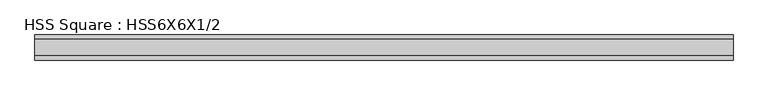
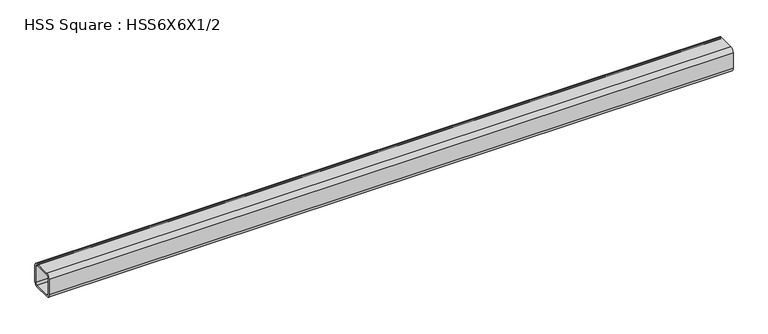
"""IFC4 building model written with IfcOpenShell, lengths in millimetres: member geometry, HSS Square : HSS6X6X1/2."""

from ifc_helpers import new_model, si_unit, point, frame, frame_2d, origin, place, context, project, spatial, polyline, circle_curve, trimmed, segment, composite_curve, outline, extrude, source, transform, mapped, element, save


def hss_square_hss6x6x1_2_c82ee425(model_context):
    return source(origin(), model_context, "Body", "SweptSolid", [
        extrude(outline(composite_curve([segment(trimmed(circle_curve(frame_2d((-50.8, 50.8)), 25.4), [point((-76.2, 50.8))], [point((-50.8, 76.2))], False, "CARTESIAN"), True, "CONTINUOUS"), segment(polyline([(-50.8, 76.2), (50.8, 76.2)]), True, "CONTINUOUS"), segment(trimmed(circle_curve(frame_2d((50.8, 50.8)), 25.4), [point((50.8, 76.2))], [point((76.2, 50.8))], False, "CARTESIAN"), True, "CONTINUOUS"), segment(polyline([(76.2, 50.8), (76.2, -50.8)]), True, "CONTINUOUS"), segment(trimmed(circle_curve(frame_2d((50.8, -50.8)), 25.4), [point((76.2, -50.8))], [point((50.8, -76.2))], False, "CARTESIAN"), True, "CONTINUOUS"), segment(polyline([(50.8, -76.2), (-50.8, -76.2)]), True, "CONTINUOUS"), segment(trimmed(circle_curve(frame_2d((-50.8, -50.8)), 25.4), [point((-50.8, -76.2))], [point((-76.2, -50.8))], False, "CARTESIAN"), True, "CONTINUOUS"), segment(polyline([(-76.2, -50.8), (-76.2, 50.8)]), True, "CONTINUOUS")], self_intersect=False), holes=[composite_curve([segment(polyline([(50.8, 63.5), (-50.8, 63.5)]), True, "CONTINUOUS"), segment(trimmed(circle_curve(frame_2d((-50.8, 50.8)), 12.7), [point((-50.8, 63.5))], [point((-63.5, 50.8))], True, "CARTESIAN"), True, "CONTINUOUS"), segment(polyline([(-63.5, 50.8), (-63.5, -50.8)]), True, "CONTINUOUS"), segment(trimmed(circle_curve(frame_2d((-50.8, -50.8)), 12.7), [point((-63.5, -50.8))], [point((-50.8, -63.5))], True, "CARTESIAN"), True, "CONTINUOUS"), segment(polyline([(-50.8, -63.5), (50.8, -63.5)]), True, "CONTINUOUS"), segment(trimmed(circle_curve(frame_2d((50.8, -50.8)), 12.7), [point((50.8, -63.5))], [point((63.5, -50.8))], True, "CARTESIAN"), True, "CONTINUOUS"), segment(polyline([(63.5, -50.8), (63.5, 50.8)]), True, "CONTINUOUS"), segment(trimmed(circle_curve(frame_2d((50.8, 50.8)), 12.7), [point((63.5, 50.8))], [point((50.8, 63.5))], True, "CARTESIAN"), True, "CONTINUOUS")], self_intersect=False)]), frame((-2089.8594122, 0.0, 0.0), z_axis=(1.0, 0.0, 0.0), x_axis=(0.0, 1.0, 0.0)), (0.0, 0.0, 1.0), 4230.3820097),
    ])


if __name__ == "__main__":
    model = new_model("IFC4")
    model_context = context("Model", 3, world=origin())
    ifc_project = project(units=[si_unit("LENGTHUNIT", "METRE", prefix="MILLI")], contexts=[model_context])
    site = spatial("IfcSite", under=ifc_project)
    building = spatial("IfcBuilding", under=site)
    placement = place(None, origin())
    hss_square_hss6x6x1_2_shape = hss_square_hss6x6x1_2_c82ee425(model_context)
    element("IfcMember", 1, ObjectType="HSS Square : HSS6X6X1/2", at=placement, inside=building, context=model_context, shape_type="MappedRepresentation", body=[
        mapped(hss_square_hss6x6x1_2_shape, transform((0.0, 0.0, 0.0), x_axis=(1.0, 0.0, 0.0), y_axis=(0.0, 1.0, 0.0), z_axis=(0.0, 0.0, 1.0))),
    ])
    save(model, "model.ifc")

# Revit data of these elements
# Type "HSS Square : HSS6X6X1/2"
#   Section Name Key = "HSS 6X6X1/2"
#   Assembly Code = "B10"
#   Width = 6.000"
#   Wall Nominal Thickness = 0.500"
#   Wall Design Thickness = 0.465"
#   Torsional Moment of Inertia = 81.10 in⁴
#   Torsional Modulus = 28.10 in³
#   Section Area = 9.74 in²
#   Plastic Modulus weak axis = 19.80 in³
#   Plastic Modulus strong axis = 19.80 in³
#   Outer Fillet = 1.000"
#   Nominal Weight = 35.24 lbf/ft
#   Moment of Inertia weak axis = 48.30 in⁴
#   Moment of Inertia strong axis = 48.30 in⁴
#   Inner Fillet = 0.500"
#   Height = 6.000"
#   Elastic Modulus weak axis = 16.10 in³
#   Elastic Modulus strong axis = 16.10 in³
#   Centroid Vertical = 3.000"
#   Centroid Horizontal = 3.000"
#   Length [instance default] = 5' - 0"
#   Structural Material [instance default] = Steel ASTM A500, Grade B, Rectangular and Square
#   Principal Axes Angle = 0
# Element 1 (IfcMember, "HSS Square : HSS6X6X1/2")
#   Structural Material = Steel ASTM A992
#   Materials on its faces: "Steel ASTM A992"
# Materials
#   "Steel ASTM A500, Grade B, Rectangular and Square": class "Metal", colour RGB 199 199 199, transparency 0, Description = "Carbon steel", Cost = 0
#   "Steel ASTM A992": class "Metal", colour RGB 199 199 199, transparency 0, Description = "Structural steel 50ksi", Cost = 0
